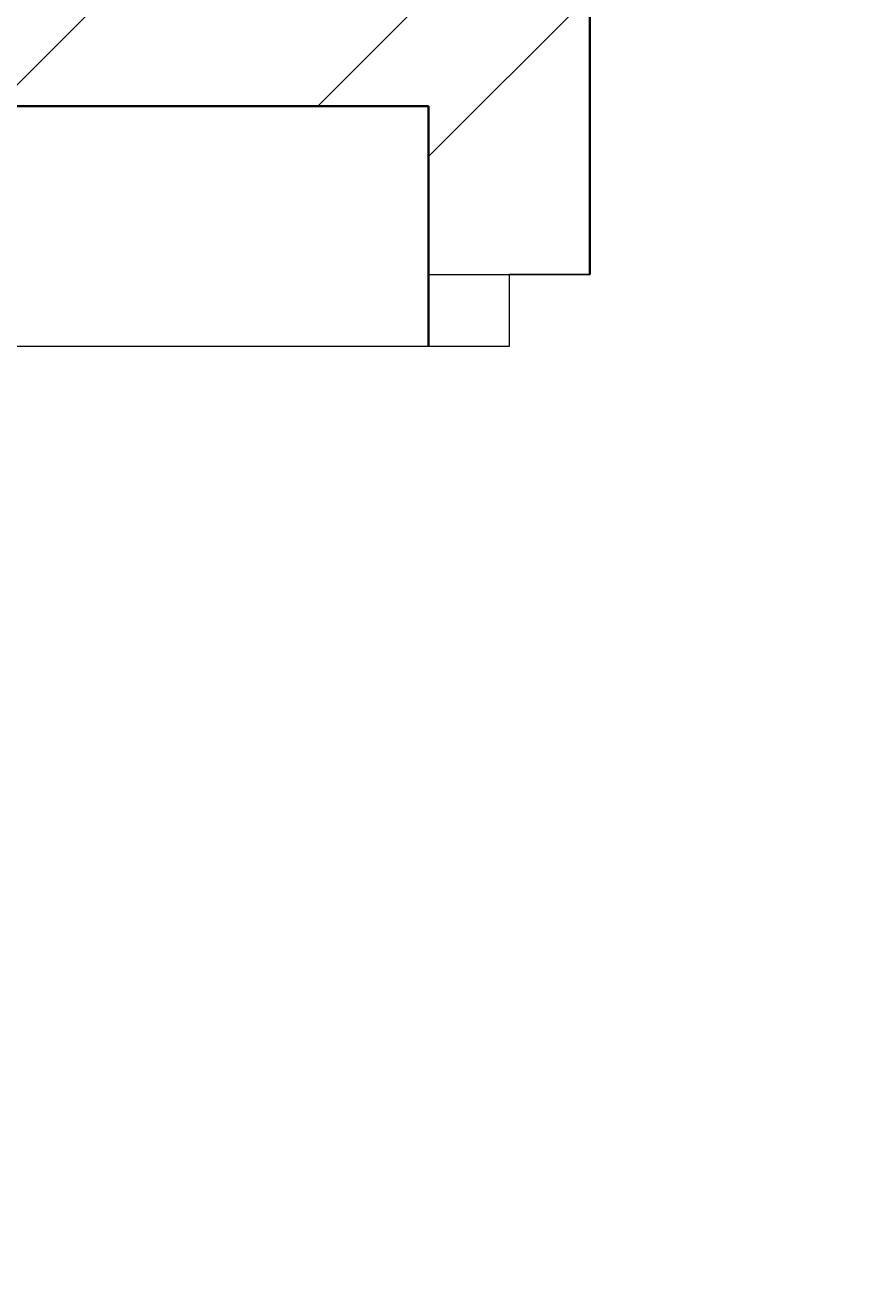
# Model space of a CAD drawing. Units: inches. Extents: x 1962 to 2771, y 1245 to 2660.
# Tile 59 of 114: x 2224 to 2247, y 2145 to 2180. Entities that reach past the tile are written whole.
import ezdxf

# ---------------------------------------------------------------- set-up
doc = ezdxf.new("R2010")
doc.units = ezdxf.units.IN
for name, color, linetype, lineweight in [('A-ANNO-DIMS', 2, 'Continuous', 18), ('A-DOOR', 3, 'Continuous', 18), ('A-WALL', 7, 'Continuous', 35), ('A-WALL-PATT', 252, 'Continuous', 13)]:
    doc.layers.add(name, color=color, linetype=linetype, lineweight=lineweight)
doc.styles.get("Standard").update_dxf_attribs({"font": 'arial.ttf'})
doc.dimstyles.get("Standard").update_dxf_attribs({"dimtxt": 0.18, "dimasz": 0.18, "dimexe": 0.18, "dimexo": 0.0625, "dimgap": 0.09, "dimtad": 0, "dimtih": 1, "dimtoh": 1, "dimdec": 4, "dimzin": 0, "dimdsep": 46, "dimtxsty": 'Standard', "dimcen": 0.09, "dimadec": 0, "dimazin": 0, "dimtfac": 1, "dimtdec": 4, "dimtofl": 0, "dimtmove": 0, "dimatfit": 3, "dimfxl": 1, "dimtolj": 1, "dimtzin": 0, "dimarcsym": 0})

# ---------------------------------------------------------------- blocks, each defined once
blk = doc.blocks.new('*D40')
at = {"layer": 'A-ANNO-DIMS', "color": 0, "lineweight": -2, "transparency": 16777216}
for p, q in [((2072.02, 2033.906), (2072.02, 2583.474)), ((2072.2, 2583.294), (2366.02, 2583.294)), ((2660.627, 2583.294), (2366.808, 2583.294)), ((2660.807, 2524.406), (2660.807, 2583.474))]:
    blk.add_line(p, q, dxfattribs=at)
at = {"layer": 'A-ANNO-DIMS', "color": 0, "transparency": 16777216}
for points in [[(2072.2, 2583.324), (2072.2, 2583.264), (2072.02, 2583.294)], [(2660.627, 2583.324), (2660.627, 2583.264), (2660.807, 2583.294)]]:
    blk.add_solid(points, dxfattribs=at)
at = {"layer": 'Defpoints', "color": 0, "transparency": 16777216}
for p in [(2660.807, 2583.294), (2660.807, 2524.344), (2072.02, 2033.844)]:
    blk.add_point(p, dxfattribs=at)
at = {"layer": 'A-ANNO-DIMS', "color": 0, "transparency": 16777216, "insert": (2366.414, 2583.294), "char_height": 0.18, "attachment_point": 5}
blk.add_mtext('\\A1;588.8', dxfattribs=at)

msp = doc.modelspace()

# ---------------------------------------------------------------- hatches: boundary and pattern name
at = {"layer": 'A-WALL-PATT'}
h = msp.add_hatch(dxfattribs=at)
h.set_pattern_fill('ANSI32', color=256)
h.paths.add_polyline_path([(2090.8074, 2467.3437), (2141.6481, 2467.3437), (2141.6481, 2469.5937), (2141.6481, 2471.8437), (2086.3074, 2471.8437), (2086.3074, 2422.5333), (2090.8074, 2422.5333)])
h.paths.add_polyline_path([(2282.7664, 2471.8437), (2204.8982, 2471.8437), (2204.8982, 2467.3437), (2234.8074, 2467.3437), (2234.8074, 2311.3437), (2228.7492, 2311.3437), (2228.7492, 2306.8437), (2234.8074, 2306.8437), (2331.9227, 2306.8437), (2331.9227, 2309.0937), (2331.9227, 2311.3437), (2239.3074, 2311.3437), (2239.3074, 2467.3437), (2282.7664, 2467.3437), (2282.7664, 2469.5937)])
h.paths.add_polyline_path([(2471.4531, 2519.8437), (2552.011, 2519.8437), (2564.3996, 2519.8437), (2564.3996, 2511.1389), (2568.8996, 2511.1389), (2568.8996, 2524.3437), (2466.9531, 2524.3437), (2466.9531, 2471.8437), (2450.0749, 2471.8437), (2446.4672, 2471.8437), (2446.4672, 2467.3437), (2450.0749, 2467.3437), (2475.9988, 2467.3437), (2475.9988, 2469.5937), (2475.9988, 2471.8437), (2471.4531, 2471.8437)])
h.paths.add_polyline_path([(2575.2231, 2469.5937), (2575.2231, 2471.8437), (2568.8996, 2471.8437), (2568.8996, 2487.1389), (2564.3996, 2487.1389), (2564.3996, 2471.8437), (2556.511, 2471.8437), (2499.2904, 2471.8437), (2499.2904, 2467.3437), (2507.8074, 2467.3437), (2507.8074, 2311.3437), (2414.863, 2311.3437), (2414.863, 2306.8437), (2512.3074, 2306.8437), (2517.0114, 2306.8437), (2517.0114, 2309.0937), (2517.0114, 2311.3437), (2512.3074, 2311.3437), (2512.3074, 2467.3437), (2575.2231, 2467.3437)])
h.paths.add_polyline_path([(2660.8074, 2471.8437), (2600.9602, 2471.8437), (2600.9602, 2467.3437), (2656.3074, 2467.3437), (2656.3074, 2432.5704), (2660.8074, 2432.5704)])
h.paths.add_polyline_path([(2660.8074, 2372.5704), (2656.3074, 2372.5704), (2656.3074, 2311.3437), (2600.276, 2311.3437), (2600.276, 2309.0937), (2600.276, 2306.8437), (2656.3074, 2306.8437), (2656.3074, 2296.2593), (2660.8074, 2296.2593)])
h.paths.add_polyline_path([(2572.3074, 2306.8437), (2577.1385, 2306.8437), (2577.1385, 2311.3437), (2551.082, 2311.3437), (2551.082, 2306.8437), (2567.8074, 2306.8437), (2567.8074, 2258.8437), (2540.0574, 2258.8437), (2540.0574, 2256.5937), (2540.0574, 2254.3437), (2567.8074, 2254.3437), (2656.3074, 2254.3437), (2656.3074, 2236.9085), (2660.8074, 2236.9085), (2660.8074, 2272.2593), (2656.3074, 2272.2593), (2656.3074, 2258.8437), (2572.3074, 2258.8437)])
h.paths.add_polyline_path([(2512.3074, 2254.3437), (2518.8716, 2254.3437), (2518.8716, 2256.5937), (2518.8716, 2258.8437), (2507.8074, 2258.8437), (2507.8074, 2177.8437), (2567.8074, 2177.8437), (2567.8074, 2172.9628), (2572.3074, 2172.9628), (2572.3074, 2177.8437), (2656.3074, 2177.8437), (2656.3074, 2166.4846), (2660.8074, 2166.4846), (2660.8074, 2200.9085), (2656.3074, 2200.9085), (2656.3074, 2182.3437), (2512.3074, 2182.3437)])
h.paths.add_polyline_path([(2656.3074, 2129.8437), (2572.3074, 2129.8437), (2572.3074, 2150.3044), (2570.0574, 2150.3044), (2567.8074, 2150.3044), (2567.8074, 2129.8437), (2507.8074, 2129.8437), (2507.8074, 2116.3027), (2510.0574, 2116.3027), (2512.3074, 2116.3027), (2512.3074, 2125.3437), (2567.8074, 2125.3437), (2572.3074, 2125.3437), (2656.3074, 2125.3437)])
h.paths.add_polyline_path([(2090.8074, 2362.5333), (2086.3074, 2362.5333), (2086.3074, 2298.6242), (2090.8074, 2298.6242), (2090.8074, 2306.8437), (2174.8074, 2306.8437), (2174.8074, 2286.4178), (2179.3074, 2286.4178), (2179.3074, 2306.8437), (2192.8641, 2306.8437), (2192.8641, 2309.0937), (2192.8641, 2311.3437), (2090.8074, 2311.3437)])
h.paths.add_polyline_path([(2209.156, 2258.8437), (2179.3074, 2258.8437), (2179.3074, 2263.2236), (2177.0574, 2263.2236), (2174.8074, 2263.2236), (2174.8074, 2258.8437), (2090.8074, 2258.8437), (2090.8074, 2274.6242), (2086.3074, 2274.6242), (2086.3074, 2238.2967), (2088.5574, 2238.2967), (2090.8074, 2238.2967), (2090.8074, 2254.3437), (2209.156, 2254.3437)])
h.paths.add_polyline_path([(2090.8074, 2177.8437), (2234.8074, 2177.8437), (2234.8074, 2173.1428), (2239.3074, 2173.1428), (2239.3074, 2258.8437), (2230.8442, 2258.8437), (2230.8442, 2256.5937), (2230.8442, 2254.3437), (2234.8074, 2254.3437), (2234.8074, 2182.3437), (2090.8074, 2182.3437), (2090.8074, 2202.2967), (2086.3074, 2202.2967), (2086.3074, 2140.0389), (2090.8074, 2140.0389)])
h.paths.add_polyline_path([(2090.8074, 2080.0389), (2086.3074, 2080.0389), (2086.3074, 2033.8437), (2090.8074, 2033.8437)], flags=17)
h.paths.add_polyline_path([(2244.9405, 2033.8437), (2239.3074, 2033.8437), (2239.3074, 2142.0665), (2237.2592, 2142.0665), (2234.8074, 2142.0665), (2234.8074, 2033.8437), (2090.8074, 2033.8437), (2076.5204, 2033.8437), (2072.0204, 2033.8437), (2072.0204, 2000.4493), (2076.5204, 2000.4493), (2076.5204, 2029.3437), (2090.8074, 2029.3437), (2244.9405, 2029.3437), (2244.9405, 2031.5937)])
h.paths.add_polyline_path([(2234.8074, 1933.3437), (2076.5204, 1933.3437), (2076.5204, 1952.4493), (2074.2704, 1952.4493), (2072.0204, 1952.4493), (2072.0204, 1933.3437), (2072.0204, 1928.8437), (2234.8074, 1928.8437)])
h.paths.add_polyline_path([(2090.8074, 1928.8437), (2086.3074, 1928.8437), (2086.3074, 1906.5013), (2090.8074, 1906.5013)])
h.paths.add_polyline_path([(2090.8074, 1846.5013), (2086.3074, 1846.5013), (2086.3074, 1769.9917), (2088.5574, 1769.9917), (2090.8074, 1769.9917), (2090.8074, 1780.3437), (2234.8074, 1780.3437), (2234.8074, 1708.3437), (2230.3764, 1708.3437), (2230.3764, 1703.8437), (2239.3074, 1703.8437), (2239.3074, 1792.6669), (2237.0574, 1792.6669), (2234.8074, 1792.6669), (2234.8074, 1784.8437), (2090.8074, 1784.8437)])
h.paths.add_polyline_path([(2239.3074, 1928.8437), (2244.9405, 1928.8437), (2244.9405, 1931.0937), (2244.9405, 1933.3437), (2234.8074, 1933.3437), (2234.8074, 1928.8437), (2234.8074, 1825.5949), (2239.3074, 1825.5949)])
h.paths.add_polyline_path([(2148.0425, 1649.0937), (2148.0425, 1651.3437), (2090.8074, 1651.3437), (2090.8074, 1646.8437), (2148.0425, 1646.8437)], flags=0)
h.paths.add_polyline_path([(2207.5601, 1708.3437), (2090.8074, 1708.3437), (2090.8074, 1703.8437), (2174.8074, 1703.8437), (2174.8074, 1651.3437), (2170.4457, 1651.3437), (2170.4457, 1646.8437), (2195.9924, 1646.8437), (2195.9924, 1649.0937), (2195.9924, 1651.3437), (2179.3074, 1651.3437), (2179.3074, 1703.8437), (2207.5601, 1703.8437), (2207.5601, 1706.0937)])
h.paths.add_polyline_path([(2090.8074, 1733.9917), (2086.3074, 1733.9917), (2086.3074, 1696.1032), (2088.5574, 1696.1032), (2090.8074, 1696.1032)])
h.paths.add_polyline_path([(2090.8074, 1672.1032), (2086.3074, 1672.1032), (2086.3074, 1600.3335), (2090.8074, 1600.3335)])
h.paths.add_polyline_path([(2090.8074, 1540.3335), (2086.3074, 1540.3335), (2086.3074, 1486.3437), (2139.6766, 1486.3437), (2139.6766, 1490.8437), (2090.8074, 1490.8437)])
h.paths.add_polyline_path([(2302.3876, 1490.8437), (2239.3074, 1490.8437), (2239.3074, 1646.8437), (2335.9994, 1646.8437), (2335.9994, 1651.3437), (2229.884, 1651.3437), (2229.884, 1646.8437), (2234.8074, 1646.8437), (2234.8074, 1490.8437), (2202.7103, 1490.8437), (2202.7103, 1488.5937), (2202.7103, 1486.3437), (2275.0699, 1486.3437), (2275.0699, 1475.772), (2279.5699, 1475.772), (2279.5699, 1486.3437), (2302.3876, 1486.3437)])
h.paths.add_polyline_path([(2279.5699, 1451.772), (2275.0699, 1451.772), (2275.0699, 1438.3437), (2174.8074, 1438.3437), (2174.8074, 1486.3437), (2179.7922, 1486.3437), (2179.7922, 1490.8437), (2163.3585, 1490.8437), (2163.3585, 1488.5937), (2163.3585, 1486.3437), (2170.3074, 1486.3437), (2170.3074, 1433.8437), (2279.5699, 1433.8437)])
h.paths.add_polyline_path([(2427.2363, 1490.8437), (2375.8074, 1490.8437), (2375.8074, 1646.8437), (2381.6401, 1646.8437), (2381.6401, 1651.3437), (2365.887, 1651.3437), (2365.887, 1649.0937), (2365.887, 1646.8437), (2371.3074, 1646.8437), (2371.3074, 1490.8437), (2327.5627, 1490.8437), (2327.5627, 1488.5937), (2327.5627, 1486.3437), (2371.3074, 1486.3437), (2371.3074, 1433.8437), (2375.8074, 1433.8437), (2375.8074, 1486.3437), (2427.2363, 1486.3437)])
h.paths.add_polyline_path([(2512.3074, 1646.8437), (2519.4351, 1646.8437), (2519.4351, 1649.0937), (2519.4351, 1651.3437), (2507.8074, 1651.3437), (2416.0063, 1651.3437), (2416.0063, 1649.0937), (2416.0063, 1646.8437), (2507.8074, 1646.8437), (2507.8074, 1490.8437), (2497.0532, 1490.8437), (2497.0532, 1488.5937), (2497.0532, 1486.3437), (2574.9344, 1486.3437), (2574.9344, 1476.0181), (2579.4344, 1476.0181), (2579.4344, 1486.3437), (2584.4872, 1486.3437), (2584.3074, 1490.8437), (2512.3074, 1490.8437)])
h.paths.add_polyline_path([(2470.5091, 1486.3437), (2473.9767, 1486.3437), (2473.9767, 1490.8437), (2449.6605, 1490.8437), (2449.6605, 1488.5937), (2449.6605, 1486.3437), (2466.0091, 1486.3437), (2466.0091, 1433.8437), (2470.5091, 1433.8437), (2579.4344, 1433.8437), (2579.4344, 1452.0181), (2574.9344, 1452.0181), (2574.9344, 1438.3437), (2554.5091, 1438.3437), (2470.5091, 1438.3437)])
h.paths.add_polyline_path([(2656.3074, 1490.8437), (2611.86, 1490.8437), (2611.86, 1486.3437), (2656.3074, 1486.3437)])
h.paths.add_polyline_path([(2660.8074, 1532.7007), (2658.5574, 1532.7007), (2656.3074, 1532.7007), (2656.3074, 1486.3437), (2660.8074, 1486.3437)])
h.paths.add_polyline_path([(2660.8074, 1664.9663), (2656.3074, 1664.9663), (2656.3074, 1651.3437), (2602.2313, 1651.3437), (2602.2313, 1646.8437), (2656.3074, 1646.8437), (2656.3074, 1592.7007), (2660.8074, 1592.7007)])
h.paths.add_polyline_path([(2660.8074, 1724.5221), (2656.3074, 1724.5221), (2656.3074, 1703.8437), (2542.4725, 1703.8437), (2542.4725, 1699.3437), (2567.8074, 1699.3437), (2567.8074, 1651.3437), (2552.7766, 1651.3437), (2552.7766, 1649.0937), (2552.7766, 1646.8437), (2577.2878, 1646.8437), (2577.2878, 1649.0937), (2577.2878, 1651.3437), (2572.3074, 1651.3437), (2572.3074, 1699.3437), (2656.3074, 1699.3437), (2656.3074, 1688.9663), (2660.8074, 1688.9663)])
h.paths.add_polyline_path([(2660.8074, 1880.6524), (2656.3074, 1880.6524), (2656.3074, 1832.8437), (2512.3074, 1832.8437), (2512.3074, 1837.8959), (2507.8074, 1837.8959), (2507.8074, 1828.3437), (2567.8074, 1828.3437), (2567.8074, 1804.3437), (2572.3074, 1804.3437), (2572.3074, 1828.3437), (2656.3074, 1828.3437), (2656.3074, 1818.6778), (2660.8074, 1818.6778)])
h.paths.add_polyline_path([(2660.8074, 1794.6778), (2656.3074, 1794.6778), (2656.3074, 1780.3437), (2572.3074, 1780.3437), (2572.3074, 1783.0303), (2570.0574, 1783.0303), (2567.8074, 1783.0303), (2567.8074, 1780.3437), (2507.8074, 1780.3437), (2507.8074, 1699.3437), (2517.8858, 1699.3437), (2517.8858, 1701.5937), (2517.8858, 1703.8437), (2512.3074, 1703.8437), (2512.3074, 1775.8437), (2656.3074, 1775.8437), (2656.3074, 1760.5221), (2660.8074, 1760.5221)])
h.paths.add_polyline_path([(2660.8074, 1981.3437), (2660.8074, 2020.2808), (2658.5574, 2020.2808), (2656.3074, 2020.2808), (2656.3074, 1981.3437), (2512.3074, 1981.3437), (2512.3074, 2086.6996), (2507.8074, 2086.6996), (2507.8074, 1981.3437), (2375.8074, 1981.3437), (2375.8074, 1986.8505), (2373.5574, 1986.8505), (2371.3074, 1986.8505), (2371.3074, 1973.2607), (2375.8074, 1973.2607), (2375.8074, 1976.8437), (2507.8074, 1976.8437), (2507.8074, 1865.4281), (2510.0574, 1865.4281), (2512.3074, 1865.4281), (2512.3074, 1976.8437), (2660.8074, 1976.8437)])
h.paths.add_polyline_path([(2375.8074, 1940.297), (2373.5574, 1940.297), (2371.3074, 1940.297), (2371.3074, 1933.3437), (2278.4434, 1933.3437), (2278.4434, 1928.8437), (2371.3074, 1928.8437), (2371.3074, 1651.3437), (2375.8074, 1651.3437)])
h.paths.add_polyline_path([(2660.8074, 1976.8437), (2656.3074, 1976.8437), (2656.3074, 1940.6524), (2660.8074, 1940.6524)], flags=17)
h.paths.add_polyline_path([(2660.8074, 2142.4846), (2656.3074, 2142.4846), (2656.3074, 2080.2808), (2660.8074, 2080.2808)])
h.paths.add_polyline_path([(2381.4189, 2311.3437), (2375.8074, 2311.3437), (2375.8074, 2467.3437), (2424.7242, 2467.3437), (2424.7242, 2469.5937), (2424.7242, 2471.8437), (2375.8074, 2471.8437), (2375.8074, 2524.3437), (2371.3074, 2524.3437), (2371.3074, 2471.8437), (2307.2097, 2471.8437), (2307.2097, 2467.3437), (2371.3074, 2467.3437), (2371.3074, 2311.3437), (2366.8901, 2311.3437), (2366.8901, 2306.8437), (2371.3074, 2306.8437), (2371.3074, 2033.8437), (2279.6589, 2033.8437), (2279.6589, 2029.3437), (2371.3074, 2029.3437), (2371.3074, 2014.2598), (2375.8074, 2014.2598), (2375.8074, 2306.8437), (2381.4189, 2306.8437)])
h.paths.add_polyline_path([(2263.3074, 2524.3437), (2170.3074, 2524.3437), (2170.3074, 2519.8437), (2170.3074, 2471.8437), (2165.0312, 2471.8437), (2165.0312, 2467.3437), (2179.6721, 2467.3437), (2179.6721, 2469.5161), (2179.6721, 2471.8437), (2174.8074, 2471.8437), (2174.8074, 2519.8437), (2258.8074, 2519.8437), (2258.8074, 2511.6436), (2263.3074, 2511.6436)])
h.paths.add_polyline_path([(2245.0232, 1361.4123), (2492.9468, 1361.4123), (2492.9468, 1398.505), (2245.0232, 1398.505)], flags=9)
h.paths.add_polyline_path([(2388.1434, 2086.6936), (2425.0704, 2086.6936), (2425.0704, 2105.3509), (2388.1434, 2105.3509)], flags=9)
h.paths.add_polyline_path([(2404.922, 2242.6744), (2445.7337, 2242.6744), (2445.7337, 2261.3318), (2404.922, 2261.3318)], flags=9)
h.paths.add_polyline_path([(2269.4107, 2156.7935), (2306.3378, 2156.7935), (2306.3378, 2175.4508), (2269.4107, 2175.4508)], flags=9)
h.paths.add_polyline_path([(2269.3277, 2233.4343), (2306.2547, 2233.4343), (2306.2547, 2252.0917), (2269.3277, 2252.0917)], flags=9)
h.paths.add_polyline_path([(2431.6052, 2320.6922), (2470.4456, 2320.6922), (2470.4456, 2339.3495), (2431.6052, 2339.3495)], flags=25)
h.paths.add_polyline_path([(2249.6902, 2315.7608), (2288.5306, 2315.7608), (2288.5306, 2334.4182), (2249.6902, 2334.4182)], flags=25)
h.paths.add_polyline_path([(2096.9301, 2314.3181), (2135.7704, 2314.3181), (2135.7704, 2332.9755), (2096.9301, 2332.9755)], flags=25)
h.paths.add_polyline_path([(2134.3475, 2285.7089), (2161.4655, 2285.7089), (2161.4655, 2304.3662), (2134.3475, 2304.3662)], flags=9)
h.paths.add_polyline_path([(2126.5155, 2209.4076), (2159.9227, 2209.4076), (2159.9227, 2228.065), (2126.5155, 2228.065)], flags=25)
h.paths.add_polyline_path([(2110.5753, 2141.5299), (2149.4157, 2141.5299), (2149.4157, 2160.1872), (2110.5753, 2160.1872)], flags=25)
h.paths.add_polyline_path([(2249.8618, 1968.3317), (2286.3966, 1968.3317), (2286.3966, 1986.989), (2249.8618, 1986.989)], flags=9)
h.paths.add_polyline_path([(2395.9507, 1777.0051), (2436.7624, 1777.0051), (2436.7624, 1795.6625), (2395.9507, 1795.6625)], flags=9)
h.paths.add_polyline_path([(2398.5259, 1888.5651), (2435.0062, 1888.5651), (2435.0062, 1907.2224), (2398.5259, 1907.2224)], flags=25)
h.paths.add_polyline_path([(2259.3506, 1728.3559), (2296.2776, 1728.3559), (2296.2776, 1747.0132), (2259.3506, 1747.0132)], flags=9)
h.paths.add_polyline_path([(2271.3698, 1845.268), (2308.2968, 1845.268), (2308.2968, 1863.9253), (2271.3698, 1863.9253)], flags=9)
h.paths.add_polyline_path([(2120.9355, 1786.3027), (2159.7759, 1786.3027), (2159.7759, 1804.9601), (2120.9355, 1804.9601)], flags=25)
h.paths.add_polyline_path([(2121.3164, 1732.1043), (2154.7236, 1732.1043), (2154.7236, 1750.7616), (2121.3164, 1750.7616)], flags=25)
h.paths.add_polyline_path([(2118.3706, 1678.8997), (2147.5282, 1678.8997), (2147.5282, 1697.557), (2118.3706, 1697.557)], flags=25)
h.paths.add_polyline_path([(2385.9227, 1493.557), (2424.763, 1493.557), (2424.763, 1512.2143), (2385.9227, 1512.2143)], flags=25)
h.paths.add_polyline_path([(2248.7058, 1500.0256), (2287.5462, 1500.0256), (2287.5462, 1518.6829), (2248.7058, 1518.6829)], flags=25)
h.paths.add_polyline_path([(2104.1669, 1617.3771), (2143.0073, 1617.3771), (2143.0073, 1636.0344), (2104.1669, 1636.0344)], flags=9)
h.paths.add_polyline_path([(2096.0714, 1447.8824), (2137.3845, 1447.8824), (2137.3845, 1458.1859), (2096.0714, 1458.1859)], flags=9)
h.paths.add_polyline_path([(2180.6114, 1440.325), (2209.7689, 1440.325), (2209.7689, 1458.9823), (2180.6114, 1458.9823)], flags=25)
h.paths.add_polyline_path([(2316.1698, 1447.9637), (2357.4829, 1447.9637), (2357.4829, 1458.2673), (2316.1698, 1458.2673)], flags=9)
h.paths.add_polyline_path([(2397.6187, 1447.9637), (2438.9318, 1447.9637), (2438.9318, 1458.2673), (2397.6187, 1458.2673)], flags=9)
h.paths.add_polyline_path([(2473.0778, 1439.5953), (2502.2354, 1439.5953), (2502.2354, 1458.2527), (2473.0778, 1458.2527)], flags=25)
h.paths.add_polyline_path([(2589.7027, 1447.8819), (2631.0158, 1447.8819), (2631.0158, 1458.1855), (2589.7027, 1458.1855)], flags=9)
h.paths.add_polyline_path([(2522.4009, 1497.5285), (2561.2413, 1497.5285), (2561.2413, 1516.1859), (2522.4009, 1516.1859)], flags=25)
h.paths.add_polyline_path([(2579.6565, 1671.3482), (2608.8141, 1671.3482), (2608.8141, 1690.0056), (2579.6565, 1690.0056)], flags=25)
h.paths.add_polyline_path([(2544.7038, 1725.5064), (2578.1111, 1725.5064), (2578.1111, 1744.1637), (2544.7038, 1744.1637)], flags=25)
h.paths.add_polyline_path([(2578.1191, 1807.472), (2607.2766, 1807.472), (2607.2766, 1826.1293), (2578.1191, 1826.1293)], flags=25)
h.paths.add_polyline_path([(2595.0614, 1835.1839), (2633.9018, 1835.1839), (2633.9018, 1853.8413), (2595.0614, 1853.8413)], flags=25)
h.paths.add_polyline_path([(2567.0097, 2097.7035), (2605.8501, 2097.7035), (2605.8501, 2116.3609), (2567.0097, 2116.3609)], flags=9)
h.paths.add_polyline_path([(2586.644, 2134.6454), (2615.8015, 2134.6454), (2615.8015, 2153.3027), (2586.644, 2153.3027)], flags=9)
h.paths.add_polyline_path([(2544.6185, 2212.6783), (2578.0258, 2212.6783), (2578.0258, 2231.3356), (2544.6185, 2231.3356)], flags=25)
h.paths.add_polyline_path([(2577.0273, 2256.9023), (2606.1849, 2256.9023), (2606.1849, 2275.5597), (2577.0273, 2275.5597)], flags=24)
h.paths.add_polyline_path([(2605.2683, 2315.2821), (2644.1087, 2315.2821), (2644.1087, 2333.9395), (2605.2683, 2333.9395)], flags=25)
h.paths.add_polyline_path([(2583.1244, 2496.1815), (2624.4375, 2496.1815), (2624.4375, 2506.4851), (2583.1244, 2506.4851)], flags=9)
h.paths.add_polyline_path([(2474.761, 2497.0823), (2503.9185, 2497.0823), (2503.9185, 2515.7397), (2474.761, 2515.7397)], flags=25)
h.paths.add_polyline_path([(2387.5787, 2494.2563), (2428.902, 2494.2563), (2428.902, 2504.5598), (2387.5787, 2504.5598)], flags=9)
h.paths.add_polyline_path([(2300.1657, 2500.1564), (2341.4788, 2500.1564), (2341.4788, 2510.46), (2300.1657, 2510.46)], flags=25)
h.paths.add_polyline_path([(2176.8589, 2497.5843), (2206.0165, 2497.5843), (2206.0165, 2516.2416), (2176.8589, 2516.2416)], flags=25)
h.paths.add_polyline_path([(2097.4668, 2494.9762), (2138.7799, 2494.9762), (2138.7799, 2505.2798), (2097.4668, 2505.2798)], flags=9)

# ---------------------------------------------------------------- linework, layer by layer
at = {"layer": 'A-DOOR'}
for p, q in [((2234.8074, 2173.1428), (2239.3074, 2173.1428)), ((2239.3074, 2173.1428), (2237.0574, 2173.1428)), ((2237.0574, 2173.1428), (2237.0574, 2171.1428)), ((2237.0574, 2171.1428), (2201.0574, 2171.1428))]:
    msp.add_line(p, q, dxfattribs=at)
msp.add_arc((2229.2838, 2171.1428), 28.2264, 180, 286.41252, dxfattribs=at)
at = {"layer": 'A-WALL'}
for p, q in [((2239.3074, 2258.8437), (2239.3074, 2173.1428)), ((2090.8074, 2177.8437), (2234.8074, 2177.8437)), ((2234.8074, 2177.8437), (2234.8074, 2171.1428))]:
    msp.add_line(p, q, dxfattribs=at)

# ---------------------------------------------------------------- dimensions: what is measured, and where the dimension line sits
at = {"layer": 'A-ANNO-DIMS'}
dim = msp.add_linear_dim(base=(2660.8074, 2583.2937), p1=(2072.0204, 2033.8437), p2=(2660.8074, 2524.3437), dimstyle='Standard', override={"dimdec": 1, "dimlfac": 1, "dimrnd": 0, "dimzin": 0, "dimdsep": 46, "dimlunit": 2}, dxfattribs=at)
dim.commit()
dim.dimension.update_dxf_attribs({"geometry": '*D40', "text_midpoint": (2366.4139, 2583.2937)})

doc.saveas('drawing.dxf')
